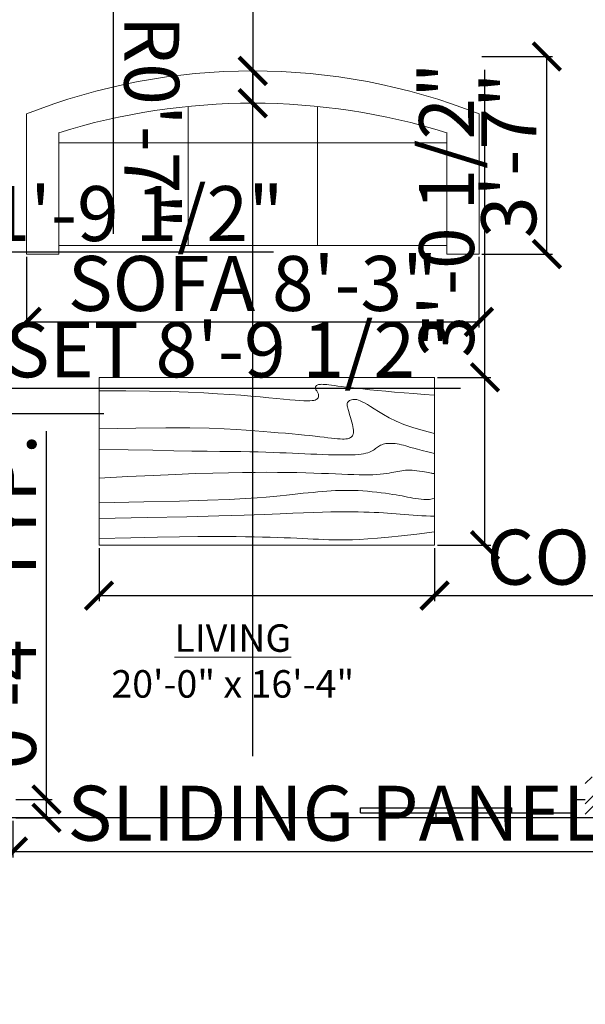
# Model space of a CAD drawing. Units: inches. Extents: x 982 to 1904, y 735 to 1463.
# Tile 5 of 7: x 1566 to 1689, y 945 to 1160. Entities that reach past the tile are written whole.
import ezdxf

# ---------------------------------------------------------------- set-up
doc = ezdxf.new("R2010")
doc.units = ezdxf.units.IN
for name, color, linetype, lineweight in [('A-AREA-IDEN', 7, 'Continuous', 18), ('A-FLOR', 7, 'Continuous', 25), ('Dimensions', 9, 'Continuous', 18), ('Doors', 130, 'Continuous', 25), ('Furniture', 31, 'Continuous', 18), ('Wall Hatch', 23, 'Continuous', 13)]:
    doc.layers.add(name, color=color, linetype=linetype, lineweight=lineweight)
doc.styles.get("Standard").update_dxf_attribs({"font": 'arial.ttf'})
doc.dimstyles.new('ISO-25', dxfattribs={"dimtxt": 12, "dimasz": 6, "dimexe": 1.25, "dimexo": 0.625, "dimtad": 1, "dimlunit": 3, "dimtxsty": 'Standard', "dimblk": 'ARCHTICK', "dimcen": 2.5, "dimadec": 0, "dimazin": 0, "dimtfac": 1, "dimtmove": 0, "dimatfit": 3, "dimfxl": 1, "dimarcsym": 0})

# ---------------------------------------------------------------- blocks, each defined once
blk = doc.blocks.new('Sofa - Roundback 7 ft.')
for p, q in [((-12.00002, -32.4421), (-12.00003, -6.5971)), ((11.99997, -32.4421), (11.99998, -6.5971)), ((-36.000027, -34), (-36.000027, -11.4696)), ((35.99998, -34), (35.99998, -11.4696)), ((-35.999844, -13.3819), (35.9998, -13.3819)), ((-36.000027, -32.4421), (35.99998, -32.4421))]:
    blk.add_line(p, q)
for points in [[(-36.000027, -34), (-42.000027, -34), (-42.000027, -8)], [(41.99998, -8), (41.99998, -34), (35.99998, -34)]]:
    blk.add_lwpolyline(points)
for centre, radius, start, end in [((0, -114.25), 114.25, 68.43141, 111.5686), ((-0.00001, -127.1968), 121.1968, 72.72033, 107.2797)]:
    blk.add_arc(centre, radius, start, end)
blk = doc.blocks.new('Table - Rectangular Woodgrain 60 x 30 in.')
for p, q in [((0, 0), (0, -30)), ((60, 0), (0, 0)), ((60, -30), (60, 0)), ((0, -30), (60, -30))]:
    blk.add_line(p, q)
for points in [[(0, -2.4), (4.8155, -2.418), (9.0302, -2.4688), (12.709, -2.5477), (15.9167, -2.65), (18.7181, -2.7711), (21.1781, -2.9063), (23.3616, -3.0508), (25.3333, -3.2), (27.1477, -3.3495), (28.8172, -3.4958), (30.3437, -3.636), (31.7291, -3.7667), (32.9756, -3.8849), (34.0849, -3.9875), (35.059, -4.0714), (35.9, -4.1334), (36.6114, -4.1711), (37.2041, -4.1854), (37.6906, -4.1779), (38.0833, -4.15), (38.3948, -4.1034), (38.6375, -4.0396), (38.8239, -3.9602), (38.9666, -3.8667), (39.0764, -3.7608), (39.1573, -3.6448), (39.2116, -3.521), (39.2416, -3.3917), (39.2498, -3.2593), (39.2385, -3.1261), (39.21, -2.9944), (39.1666, -2.8667), (39.111, -2.7447), (39.0468, -2.6281), (38.978, -2.5163), (38.9083, -2.4083), (38.8418, -2.3035), (38.7823, -2.201), (38.7337, -2.1001), (38.7, -2), (38.6844, -1.9003), (38.6875, -1.8021), (38.7094, -1.707), (38.75, -1.6167), (38.8094, -1.5326), (38.8875, -1.4563), (38.9844, -1.3893), (39.1, -1.3333), (39.2351, -1.2896), (39.3937, -1.2583), (39.5804, -1.2396), (39.8, -1.2333), (40.057, -1.2396), (40.3562, -1.2583), (40.7023, -1.2896), (41.1, -1.3333), (41.5547, -1.3895), (42.0755, -1.4573), (42.6721, -1.5361), (43.3542, -1.625), (44.1316, -1.7233), (45.014, -1.8302), (46.0114, -1.9449), (47.1333, -2.0667), (48.3862, -2.1947), (49.7625, -2.3281), (51.2513, -2.4663), (52.8416, -2.6083), (54.5226, -2.7535), (56.2833, -2.9011), (58.1127, -3.0501), (60, -3.2)], [(0, -9.2), (6.5759, -9.0858), (11.9385, -9.0365), (16.2527, -9.0418), (19.6833, -9.0917), (22.3952, -9.1759), (24.5531, -9.2844), (26.322, -9.4069), (27.8666, -9.5333), (29.3241, -9.6553), (30.7203, -9.7719), (32.0532, -9.8837), (33.3208, -9.9917), (34.5213, -10.0965), (35.6526, -10.199), (36.7128, -10.2999), (37.7, -10.4), (38.6129, -10.4996), (39.4531, -10.5969), (40.223, -10.6895), (40.925, -10.775), (41.5613, -10.8512), (42.1344, -10.9156), (42.6465, -10.966), (43.1, -11), (43.4976, -11.0158), (43.8437, -11.0136), (44.143, -10.9942), (44.4, -10.9583), (44.6195, -10.9069), (44.8062, -10.8406), (44.9648, -10.7603), (45.1, -10.6667), (45.2155, -10.5598), (45.3114, -10.4365), (45.3871, -10.2929), (45.4416, -10.125), (45.4743, -9.929), (45.4844, -9.7011), (45.4709, -9.4371), (45.4333, -9.1333), (45.3716, -8.7883), (45.2896, -8.4104), (45.1919, -8.0107), (45.0833, -7.6), (44.9685, -7.1893), (44.8521, -6.7896), (44.7388, -6.4117), (44.6333, -6.0667), (44.54, -5.7628), (44.4614, -5.4979), (44.4001, -5.2675), (44.3583, -5.0667), (44.3384, -4.8909), (44.3427, -4.7354), (44.3736, -4.5956), (44.4333, -4.4667), (44.5236, -4.3453), (44.6427, -4.2333), (44.7884, -4.1339), (44.9583, -4.05), (45.1501, -3.9849), (45.3614, -3.9417), (45.59, -3.9234), (45.8333, -3.9333), (46.0915, -3.9749), (46.3734, -4.0531), (46.6906, -4.1736), (47.0542, -4.3417), (47.4756, -4.5629), (47.9661, -4.8427), (48.5372, -5.1866), (49.2, -5.6), (49.9676, -6.0844), (50.8594, -6.625), (51.8965, -7.2031), (53.1, -7.8), (54.491, -8.3969), (56.0906, -8.975), (57.9199, -9.5156), (60, -10)], [(0, -12.8), (5.1847, -12.9322), (9.6213, -13.0323), (13.3963, -13.1059), (16.5958, -13.1583), (19.3063, -13.1952), (21.614, -13.2219), (23.6054, -13.2439), (25.3666, -13.2667), (26.9728, -13.2947), (28.4531, -13.3281), (29.8256, -13.3663), (31.1083, -13.4083), (32.3191, -13.4535), (33.476, -13.501), (34.597, -13.5501), (35.7, -13.6), (36.7984, -13.6497), (37.8875, -13.6979), (38.9578, -13.743), (40, -13.7833), (41.0047, -13.8174), (41.9625, -13.8438), (42.864, -13.8607), (43.7, -13.8667), (44.4631, -13.8604), (45.1552, -13.8417), (45.7801, -13.8104), (46.3416, -13.7667), (46.8439, -13.7104), (47.2906, -13.6417), (47.6858, -13.5604), (48.0333, -13.4667), (48.3375, -13.3608), (48.6042, -13.2448), (48.8396, -13.121), (49.05, -12.9917), (49.2417, -12.8593), (49.4208, -12.7261), (49.5937, -12.5944), (49.7667, -12.4667), (49.9452, -12.3451), (50.1323, -12.2313), (50.3303, -12.1268), (50.5416, -12.0333), (50.7686, -11.9524), (51.0135, -11.8854), (51.2788, -11.8341), (51.5666, -11.8), (51.8785, -11.7843), (52.2116, -11.7865), (52.562, -11.8059), (52.926, -11.8417), (53.2998, -11.8931), (53.6795, -11.9594), (54.0614, -12.0397), (54.4416, -12.1333), (54.8223, -12.2401), (55.2293, -12.3625), (55.6942, -12.5037), (56.2489, -12.6667), (56.9251, -12.8547), (57.7545, -13.0708), (58.7689, -13.3182), (60, -13.6)], [(0, -18), (5.124, -17.7273), (9.6609, -17.5057), (13.6705, -17.3303), (17.2125, -17.1958), (20.3467, -17.0973), (23.1328, -17.0297), (25.6307, -16.9878), (27.9, -16.9667), (29.9928, -16.9617), (31.9302, -16.9703), (33.7254, -16.9907), (35.3917, -17.0208), (36.9423, -17.0588), (38.3906, -17.1026), (39.7499, -17.1503), (41.0333, -17.2), (42.2519, -17.2496), (43.4073, -17.2969), (44.4986, -17.3395), (45.525, -17.375), (46.4858, -17.4012), (47.3802, -17.4156), (48.2074, -17.416), (48.9667, -17.4), (49.6583, -17.3662), (50.2872, -17.3167), (50.8595, -17.2547), (51.3812, -17.1833), (51.8584, -17.1057), (52.2971, -17.025), (52.7034, -16.9443), (53.0833, -16.8667), (53.443, -16.7951), (53.789, -16.7313), (54.128, -16.6768), (54.4666, -16.6334), (54.8115, -16.6024), (55.1693, -16.5854), (55.5465, -16.5841), (55.95, -16.6), (56.3828, -16.6337), (56.8346, -16.6823), (57.2915, -16.7418), (57.7396, -16.8084), (58.165, -16.878), (58.5539, -16.9469), (58.8924, -17.0111), (59.1666, -17.0667), (59.3679, -17.1107), (59.5078, -17.1438), (59.6032, -17.1675), (59.6708, -17.1833), (59.7275, -17.193), (59.7901, -17.1979), (59.8753, -17.1998), (60, -17.2)], [(0, -22.4), (8.0098, -22.2501), (14.4094, -22.1011), (19.4168, -21.9535), (23.25, -21.8083), (26.1269, -21.6663), (28.2656, -21.5281), (29.884, -21.3947), (31.2, -21.2667), (32.3967, -21.1448), (33.5172, -21.0292), (34.5697, -20.9198), (35.5625, -20.8167), (36.5037, -20.7198), (37.4015, -20.6292), (38.2642, -20.5448), (39.1, -20.4667), (39.9164, -20.3951), (40.7187, -20.3313), (41.5117, -20.2768), (42.3, -20.2333), (43.0883, -20.2024), (43.8812, -20.1854), (44.6836, -20.1841), (45.5, -20.2), (46.3328, -20.234), (47.1747, -20.2844), (48.0163, -20.3488), (48.8479, -20.425), (49.66, -20.5106), (50.4429, -20.6031), (51.1872, -20.7004), (51.8833, -20.8), (52.5246, -20.8999), (53.1166, -20.9995), (53.6681, -21.0983), (54.1875, -21.1958), (54.6834, -21.2919), (55.1646, -21.3859), (55.6394, -21.4777), (56.1167, -21.5667), (56.6028, -21.6515), (57.0961, -21.7266), (57.5929, -21.7852), (58.0896, -21.8208), (58.5823, -21.8268), (59.0674, -21.7964), (59.5412, -21.723), (60, -21.6)], [(0, -25.2), (8.6355, -25.0504), (15.7026, -24.9031), (21.4049, -24.7606), (25.9458, -24.625), (29.529, -24.4988), (32.3578, -24.3844), (34.6359, -24.284), (36.5667, -24.2), (38.3213, -24.1341), (39.9417, -24.0854), (41.437, -24.0523), (42.8167, -24.0333), (44.0901, -24.0268), (45.2667, -24.0313), (46.3557, -24.0451), (47.3667, -24.0667), (48.309, -24.0947), (49.1928, -24.1287), (50.0284, -24.168), (50.826, -24.2125), (51.5959, -24.2617), (52.3483, -24.3151), (53.0935, -24.3725), (53.8417, -24.4334), (54.6009, -24.497), (55.3699, -24.561), (56.1454, -24.6226), (56.9239, -24.6792), (57.7021, -24.7279), (58.4764, -24.7662), (59.2435, -24.7911), (60, -24.8)], [(0, -28.8), (5.6867, -28.6681), (10.45, -28.5698), (14.407, -28.5012), (17.675, -28.4584), (20.3711, -28.4374), (22.6125, -28.4344), (24.5164, -28.4455), (26.2, -28.4667), (27.762, -28.4947), (29.2276, -28.5281), (30.6033, -28.5663), (31.8958, -28.6084), (33.1118, -28.6535), (34.2578, -28.7011), (35.3405, -28.7501), (36.3666, -28.8), (37.3443, -28.8497), (38.288, -28.8974), (39.2137, -28.9412), (40.1375, -28.9792), (41.0753, -29.0093), (42.0432, -29.0297), (43.0572, -29.0384), (44.1333, -29.0333), (45.2936, -29.0114), (46.5843, -28.9641), (48.0579, -28.8816), (49.7666, -28.7542), (51.7629, -28.5721), (54.0989, -28.3255), (56.8272, -28.0048), (60, -27.6)]]:
    blk.add_lwpolyline(points)
blk = doc.blocks.new('DOOR-SLIDING-PANEL')
for p, q in [((2, 4), (0, 4)), ((2, 0), (2, 4)), ((49.05, 2.21), (16.06, 2.21)), ((16.06, 1.11), (16.06, 2.21)), ((49.05, 1.11), (49.05, 2.21)), ((49.05, 1.11), (2, 1.11)), ((32.55, 0), (32.55, 1.11))]:
    blk.add_line(p, q)
blk = doc.blocks.new('_ArchTick')
at = {"color": 0, "linetype": 'ByBlock', "const_width": 0.15}
blk.add_lwpolyline([(-0.5, -0.5), (0.5, 0.5)], dxfattribs=at)
blk = doc.blocks.new('*D38')
at = {"layer": 'Defpoints', "color": 0, "transparency": 16777216}
for p in [(1515.5, 985.99), (1564.55, 985.99), (1564.55, 978.63)]:
    blk.add_point(p, dxfattribs=at)
at = {"layer": 'Dimensions', "color": 0, "lineweight": -2, "transparency": 16777216}
for p, q in [((1515.5, 985.37), (1515.5, 977.38)), ((1564.55, 985.37), (1564.55, 977.38)), ((1515.5, 978.63), (1564.55, 978.63)), ((1564.55, 978.63), (1776.25, 978.63))]:
    blk.add_line(p, q, dxfattribs=at)
at = {"layer": 'Dimensions', "color": 0, "lineweight": -2, "transparency": 16777216, "xscale": 6, "yscale": 6, "zscale": 6, "rotation": 180}
blk.add_blockref('_ArchTick', (1515.5, 978.63), dxfattribs=at)
at = {"layer": 'Dimensions', "color": 0, "lineweight": -2, "transparency": 16777216, "xscale": 6, "yscale": 6, "zscale": 6}
blk.add_blockref('_ArchTick', (1564.55, 978.63), dxfattribs=at)
at = {"layer": 'Dimensions', "color": 0, "transparency": 16777216, "insert": (1673.4, 985.46), "char_height": 12, "attachment_point": 5}
blk.add_mtext('SLIDING PANEL 4\'-1" TYP.', dxfattribs=at)
blk = doc.blocks.new('*D39')
at = {"layer": 'Defpoints', "color": 0, "transparency": 16777216}
for p in [(1564.55, 989.99), (1571.9, 989.99), (1564.55, 985.99)]:
    blk.add_point(p, dxfattribs=at)
at = {"layer": 'Dimensions', "color": 0, "lineweight": -2, "transparency": 16777216}
for p, q in [((1571.9, 989.99), (1571.9, 1070.39)), ((1565.17, 989.99), (1573.15, 989.99)), ((1571.9, 985.99), (1571.9, 989.99)), ((1565.17, 985.99), (1573.15, 985.99))]:
    blk.add_line(p, q, dxfattribs=at)
at = {"layer": 'Dimensions', "color": 0, "lineweight": -2, "transparency": 16777216, "xscale": 6, "yscale": 6, "zscale": 6}
for p, rotation in [((1571.9, 989.99), 90), ((1571.9, 985.99), 270)]:
    blk.add_blockref('_ArchTick', p, dxfattribs=dict(at, rotation=rotation))
at = {"layer": 'Dimensions', "color": 0, "transparency": 16777216, "insert": (1565.15, 1033.19), "char_height": 12, "attachment_point": 5, "rotation": 90}
blk.add_mtext('0\'-4" TYP.', dxfattribs=at)
blk = doc.blocks.new('*D40')
at = {"layer": 'Defpoints', "color": 0, "transparency": 16777216}
for p in [(1389.84, 1095.57), (1495.17, 1095.57), (1495.17, 1079.77)]:
    blk.add_point(p, dxfattribs=at)
at = {"layer": 'Dimensions', "color": 0, "lineweight": -2, "transparency": 16777216}
for p, q in [((1389.84, 1094.94), (1389.84, 1078.52)), ((1495.17, 1094.94), (1495.17, 1078.52)), ((1389.84, 1079.77), (1495.17, 1079.77)), ((1495.17, 1079.77), (1662.27, 1079.77))]:
    blk.add_line(p, q, dxfattribs=at)
at = {"layer": 'Dimensions', "color": 0, "lineweight": -2, "transparency": 16777216, "xscale": 6, "yscale": 6, "zscale": 6, "rotation": 180}
blk.add_blockref('_ArchTick', (1389.84, 1079.77), dxfattribs=at)
at = {"layer": 'Dimensions', "color": 0, "lineweight": -2, "transparency": 16777216, "xscale": 6, "yscale": 6, "zscale": 6}
blk.add_blockref('_ArchTick', (1495.17, 1079.77), dxfattribs=at)
at = {"layer": 'Dimensions', "color": 0, "transparency": 16777216, "insert": (1581.72, 1086.6), "char_height": 12, "attachment_point": 5}
blk.add_mtext('DINING SET 8\'-9 1/2"', dxfattribs=at)
blk = doc.blocks.new('*D42')
at = {"layer": 'Defpoints', "color": 0, "transparency": 16777216}
for p in [(1567.53, 1109.05), (1666.29, 1109.05), (1666.29, 1094.24)]:
    blk.add_point(p, dxfattribs=at)
at = {"layer": 'Dimensions', "color": 0, "lineweight": -2, "transparency": 16777216}
for p, q in [((1567.53, 1108.43), (1567.53, 1092.99)), ((1666.29, 1108.43), (1666.29, 1092.99)), ((1567.53, 1094.24), (1666.29, 1094.24))]:
    blk.add_line(p, q, dxfattribs=at)
at = {"layer": 'Dimensions', "color": 0, "lineweight": -2, "transparency": 16777216, "xscale": 6, "yscale": 6, "zscale": 6, "rotation": 180}
blk.add_blockref('_ArchTick', (1567.53, 1094.24), dxfattribs=at)
at = {"layer": 'Dimensions', "color": 0, "lineweight": -2, "transparency": 16777216, "xscale": 6, "yscale": 6, "zscale": 6}
blk.add_blockref('_ArchTick', (1666.29, 1094.24), dxfattribs=at)
at = {"layer": 'Dimensions', "color": 0, "transparency": 16777216, "insert": (1616.91, 1101.08), "char_height": 12, "attachment_point": 5}
blk.add_mtext('SOFA 8\'-3"', dxfattribs=at)
blk = doc.blocks.new('*D43')
at = {"layer": 'Defpoints', "color": 0, "transparency": 16777216}
for p in [(1666.29, 1152.16), (1681.11, 1152.16), (1666.29, 1109.05)]:
    blk.add_point(p, dxfattribs=at)
at = {"layer": 'Dimensions', "color": 0, "lineweight": -2, "transparency": 16777216}
for p, q in [((1666.92, 1152.16), (1682.36, 1152.16)), ((1681.11, 1109.05), (1681.11, 1152.16)), ((1666.92, 1109.05), (1682.36, 1109.05))]:
    blk.add_line(p, q, dxfattribs=at)
at = {"layer": 'Dimensions', "color": 0, "lineweight": -2, "transparency": 16777216, "xscale": 6, "yscale": 6, "zscale": 6}
for p, rotation in [((1681.11, 1152.16), 90), ((1681.11, 1109.05), 270)]:
    blk.add_blockref('_ArchTick', p, dxfattribs=dict(at, rotation=rotation))
at = {"layer": 'Dimensions', "color": 0, "transparency": 16777216, "insert": (1674.35, 1130.61), "char_height": 12, "attachment_point": 5, "rotation": 90}
blk.add_mtext('3\'-7"', dxfattribs=at)
blk = doc.blocks.new('*D46')
at = {"layer": 'Defpoints', "color": 0, "transparency": 16777216}
for p in [(1583.35, 1045.5), (1656.61, 1045.5), (1656.61, 1034.51)]:
    blk.add_point(p, dxfattribs=at)
at = {"layer": 'Dimensions', "color": 0, "lineweight": -2, "transparency": 16777216}
for p, q in [((1583.35, 1044.87), (1583.35, 1033.26)), ((1656.61, 1044.87), (1656.61, 1033.26)), ((1583.35, 1034.51), (1656.61, 1034.51)), ((1656.61, 1034.51), (1854, 1034.51))]:
    blk.add_line(p, q, dxfattribs=at)
at = {"layer": 'Dimensions', "color": 0, "lineweight": -2, "transparency": 16777216, "xscale": 6, "yscale": 6, "zscale": 6, "rotation": 180}
blk.add_blockref('_ArchTick', (1583.35, 1034.51), dxfattribs=at)
at = {"layer": 'Dimensions', "color": 0, "lineweight": -2, "transparency": 16777216, "xscale": 6, "yscale": 6, "zscale": 6}
blk.add_blockref('_ArchTick', (1656.61, 1034.51), dxfattribs=at)
at = {"layer": 'Dimensions', "color": 0, "transparency": 16777216, "insert": (1758.31, 1041.34), "char_height": 12, "attachment_point": 5}
blk.add_mtext('COFFEE TABLE 6\'-1 1/2"', dxfattribs=at)
blk = doc.blocks.new('*D47')
at = {"layer": 'Defpoints', "color": 0, "transparency": 16777216}
for p in [(1656.61, 1082.13), (1667.6, 1082.13), (1656.61, 1045.5)]:
    blk.add_point(p, dxfattribs=at)
at = {"layer": 'Dimensions', "color": 0, "lineweight": -2, "transparency": 16777216}
for p, q in [((1667.6, 1082.13), (1667.6, 1149.23)), ((1657.24, 1082.13), (1668.85, 1082.13)), ((1667.6, 1045.5), (1667.6, 1082.13)), ((1657.24, 1045.5), (1668.85, 1045.5))]:
    blk.add_line(p, q, dxfattribs=at)
at = {"layer": 'Dimensions', "color": 0, "lineweight": -2, "transparency": 16777216, "xscale": 6, "yscale": 6, "zscale": 6}
for p, rotation in [((1667.6, 1082.13), 90), ((1667.6, 1045.5), 270)]:
    blk.add_blockref('_ArchTick', p, dxfattribs=dict(at, rotation=rotation))
at = {"layer": 'Dimensions', "color": 0, "transparency": 16777216, "insert": (1660.77, 1118.68), "char_height": 12, "attachment_point": 5, "rotation": 90}
blk.add_mtext('3\'-0 1/2"', dxfattribs=at)
blk = doc.blocks.new('*D48')
at = {"layer": 'Defpoints', "color": 0, "transparency": 16777216}
for p in [(1555.46, 1134.17), (1558.68, 1134.17), (1555.46, 1112.72)]:
    blk.add_point(p, dxfattribs=at)
at = {"layer": 'Dimensions', "color": 0, "lineweight": -2, "transparency": 16777216}
for p, q in [((1558.68, 1134.17), (1558.68, 1298.47)), ((1556.09, 1134.17), (1559.93, 1134.17)), ((1558.68, 1112.72), (1558.68, 1134.17)), ((1556.09, 1112.72), (1559.93, 1112.72))]:
    blk.add_line(p, q, dxfattribs=at)
at = {"layer": 'Dimensions', "color": 0, "lineweight": -2, "transparency": 16777216, "xscale": 6, "yscale": 6, "zscale": 6}
for p, rotation in [((1558.68, 1134.17), 90), ((1558.68, 1112.72), 270)]:
    blk.add_blockref('_ArchTick', p, dxfattribs=dict(at, rotation=rotation))
at = {"layer": 'Dimensions', "color": 0, "transparency": 16777216, "insert": (1551.85, 1219.32), "char_height": 12, "attachment_point": 5, "rotation": 90}
blk.add_mtext('END TABLE 1\'-9 1/2"', dxfattribs=at)
blk = doc.blocks.new('*D49')
at = {"layer": 'Defpoints', "color": 0, "transparency": 16777216}
for p in [(1534.01, 1112.72), (1555.46, 1112.72), (1555.46, 1109.5)]:
    blk.add_point(p, dxfattribs=at)
at = {"layer": 'Dimensions', "color": 0, "lineweight": -2, "transparency": 16777216}
for p, q in [((1534.01, 1112.09), (1534.01, 1108.25)), ((1555.46, 1112.09), (1555.46, 1108.25)), ((1534.01, 1109.5), (1555.46, 1109.5)), ((1555.46, 1109.5), (1621.44, 1109.5))]:
    blk.add_line(p, q, dxfattribs=at)
at = {"layer": 'Dimensions', "color": 0, "lineweight": -2, "transparency": 16777216, "xscale": 6, "yscale": 6, "zscale": 6, "rotation": 180}
blk.add_blockref('_ArchTick', (1534.01, 1109.5), dxfattribs=at)
at = {"layer": 'Dimensions', "color": 0, "lineweight": -2, "transparency": 16777216, "xscale": 6, "yscale": 6, "zscale": 6}
blk.add_blockref('_ArchTick', (1555.46, 1109.5), dxfattribs=at)
at = {"layer": 'Dimensions', "color": 0, "transparency": 16777216, "insert": (1591.45, 1116.33), "char_height": 12, "attachment_point": 5}
blk.add_mtext('1\'-9 1/2"', dxfattribs=at)
blk = doc.blocks.new('*D73')
at = {"layer": 'Defpoints', "color": 0, "transparency": 16777216}
for p in [(1616.91, 1141.97), (1616.91, 999.48)]:
    blk.add_point(p, dxfattribs=at)
at = {"layer": 'Dimensions', "color": 0, "lineweight": -2, "transparency": 16777216}
for p in [(1616.91, 1273.09), (1616.91, 999.48)]:
    blk.add_line(p, (1616.91, 1141.97), dxfattribs=at)
at = {"layer": 'Dimensions', "color": 0, "lineweight": -2, "transparency": 16777216, "xscale": 6, "yscale": 6, "zscale": 6, "rotation": 269.9998576619989}
blk.add_blockref('_ArchTick', (1616.91, 1141.97), dxfattribs=at)
at = {"layer": 'Dimensions', "color": 0, "transparency": 16777216, "insert": (1610.08, 1227.47), "char_height": 12, "attachment_point": 5, "rotation": 89.9999}
blk.add_mtext('R11\'-10 1/2"', dxfattribs=at)
blk = doc.blocks.new('*D74')
at = {"layer": 'Defpoints', "color": 0, "transparency": 16777216}
for p in [(1616.91, 1149.03), (1616.91, 1014.7)]:
    blk.add_point(p, dxfattribs=at)
at = {"layer": 'Dimensions', "color": 0, "lineweight": -2, "transparency": 16777216}
for p in [(1616.91, 1270.59), (1616.91, 1014.7)]:
    blk.add_line(p, (1616.91, 1149.03), dxfattribs=at)
at = {"layer": 'Dimensions', "color": 0, "lineweight": -2, "transparency": 16777216, "xscale": 6, "yscale": 6, "zscale": 6, "rotation": 269.9998536992126}
blk.add_blockref('_ArchTick', (1616.91, 1149.03), dxfattribs=at)
at = {"layer": 'Dimensions', "color": 0, "transparency": 16777216, "insert": (1610.08, 1229.63), "char_height": 12, "attachment_point": 5, "rotation": 89.9999}
blk.add_mtext('R11\'-2 1/2"', dxfattribs=at)
blk = doc.blocks.new('*D76')
at = {"layer": 'Defpoints', "color": 0, "transparency": 16777216}
for p in [(1519.04, 1074.16), (1583.2, 1074.16)]:
    blk.add_point(p, dxfattribs=at)
at = {"layer": 'Dimensions', "color": 0, "lineweight": -2, "transparency": 16777216}
for p in [(1458.22, 1074.16), (1583.2, 1074.16)]:
    blk.add_line(p, (1519.04, 1074.16), dxfattribs=at)
at = {"layer": 'Dimensions', "color": 0, "lineweight": -2, "transparency": 16777216, "xscale": 6, "yscale": 6, "zscale": 6, "rotation": 359.9995481306522}
blk.add_blockref('_ArchTick', (1519.04, 1074.16), dxfattribs=at)
at = {"layer": 'Dimensions', "color": 0, "transparency": 16777216, "insert": (1480.54, 1080.88), "char_height": 12, "attachment_point": 5, "rotation": 359.9995}
blk.add_mtext('R5\'-4"', dxfattribs=at)
blk = doc.blocks.new('*D77')
at = {"layer": 'Defpoints', "color": 0, "transparency": 16777216}
for p in [(1525.43, 1074.16), (1584.4, 1074.16)]:
    blk.add_point(p, dxfattribs=at)
at = {"layer": 'Dimensions', "color": 0, "lineweight": -2, "transparency": 16777216}
for p in [(1459.47, 1074.16), (1584.4, 1074.16)]:
    blk.add_line(p, (1525.43, 1074.16), dxfattribs=at)
at = {"layer": 'Dimensions', "color": 0, "lineweight": -2, "transparency": 16777216, "xscale": 6, "yscale": 6, "zscale": 6, "rotation": 0.0004799085174027}
blk.add_blockref('_ArchTick', (1525.43, 1074.16), dxfattribs=at)
at = {"layer": 'Dimensions', "color": 0, "transparency": 16777216, "insert": (1486.45, 1080.81), "char_height": 12, "attachment_point": 5, "rotation": 0.0005}
blk.add_mtext('R4\'-11"', dxfattribs=at)
blk = doc.blocks.new('*D79')
at = {"layer": 'Defpoints', "color": 0, "transparency": 16777216}
for p in [(1586.55, 1203.33), (1586.55, 1196.33)]:
    blk.add_point(p, dxfattribs=at)
at = {"layer": 'Dimensions', "color": 0, "lineweight": -2, "transparency": 16777216}
for p in [(1586.55, 1203.33), (1586.55, 1113.43)]:
    blk.add_line(p, (1586.55, 1196.33), dxfattribs=at)
at = {"layer": 'Dimensions', "color": 0, "lineweight": -2, "transparency": 16777216, "xscale": 6, "yscale": 6, "zscale": 6, "rotation": 90.00372422566393}
blk.add_blockref('_ArchTick', (1586.55, 1196.33), dxfattribs=at)
at = {"layer": 'Dimensions', "color": 0, "transparency": 16777216, "insert": (1593.3, 1148.88), "char_height": 12, "attachment_point": 5, "rotation": 270.0037}
blk.add_mtext('4X R0\'-7"', dxfattribs=at)

msp = doc.modelspace()

# ---------------------------------------------------------------- hatches: boundary and pattern name
at = {"layer": 'Wall Hatch'}
h = msp.add_hatch(dxfattribs=at)
h.set_pattern_fill('ANSI32', color=256, scale=0.5)
h.paths.add_polyline_path([(1165.496, 1065.991), (1271.496, 1065.991), (1271.496, 1071.991), (1218.496, 1071.991), (1218.496, 1238.491), (1262.496, 1238.491), (1262.496, 1244.491), (1218.496, 1244.491), (1218.496, 1330.491), (1298.496, 1330.491), (1298.496, 1244.491), (1292.496, 1244.491), (1292.496, 1238.491), (1298.496, 1238.491), (1298.496, 1221.991), (1304.496, 1221.991), (1304.496, 1224.991), (1374.496, 1224.991), (1374.496, 1230.991), (1304.496, 1230.991), (1304.496, 1251.991), (1310.496, 1251.991), (1310.496, 1257.991), (1304.496, 1257.991), (1304.496, 1385.991), (1328.496, 1385.991), (1328.496, 1394.991), (1295.496, 1394.991), (1295.496, 1339.491), (1209.496, 1339.491), (1209.496, 1071.991), (1156.496, 1071.991), (1156.496, 893.991), (1171.496, 893.991), (1171.496, 902.991), (1165.496, 902.991)])
h.paths.add_polyline_path([(1273.996, 877.991), (1267.996, 877.991), (1267.996, 902.991), (1252.996, 902.991), (1252.996, 893.991), (1258.996, 893.991), (1258.996, 868.991), (1273.996, 868.991)])
h.paths.add_polyline_path([(1370.496, 1052.991), (1361.496, 1052.991), (1361.496, 1046.991), (1355.496, 1046.991), (1355.496, 1040.991), (1361.496, 1040.991), (1361.496, 877.991), (1355.496, 877.991), (1355.496, 868.991), (1361.496, 868.991), (1361.496, 832.991), (1376.313, 832.991), (1491.496, 832.991), (1491.496, 985.991), (1515.496, 985.991), (1515.496, 994.991), (1482.496, 994.991), (1482.496, 841.991), (1370.496, 841.991)])
h.paths.add_polyline_path([(1319.496, 1088.991), (1325.496, 1088.991), (1325.496, 1094.991), (1319.496, 1094.991), (1319.496, 1112.491), (1361.496, 1112.491), (1361.496, 1094.991), (1355.496, 1094.991), (1355.496, 1088.991), (1361.496, 1088.991), (1361.496, 1082.991), (1370.496, 1082.991), (1370.496, 1180.991), (1503.496, 1180.991), (1503.496, 1231.991), (1497.496, 1231.991), (1497.496, 1215.991), (1491.496, 1215.991), (1491.496, 1209.991), (1497.496, 1209.991), (1497.496, 1189.991), (1448.496, 1189.991), (1448.496, 1209.991), (1454.496, 1209.991), (1454.496, 1215.991), (1448.496, 1215.991), (1448.496, 1221.991), (1442.496, 1221.991), (1442.496, 1189.991), (1380.496, 1189.991), (1380.496, 1251.991), (1442.496, 1251.991), (1442.496, 1245.991), (1448.496, 1245.991), (1448.496, 1263.991), (1442.496, 1263.991), (1442.496, 1257.991), (1368.496, 1257.991), (1368.496, 1251.991), (1374.496, 1251.991), (1374.496, 1189.991), (1304.496, 1189.991), (1304.496, 1192.991), (1295.496, 1192.991), (1295.496, 1183.991), (1361.496, 1183.991), (1361.496, 1118.491), (1313.496, 1118.491), (1313.496, 1071.991), (1301.496, 1071.991), (1301.496, 1065.991), (1313.496, 1065.991), (1313.496, 1040.991), (1325.496, 1040.991), (1325.496, 1046.991), (1319.496, 1046.991)])
h.paths.add_polyline_path([(1565.496, 1394.991), (1418.496, 1394.991), (1418.496, 1385.991), (1442.496, 1385.991), (1442.496, 1293.991), (1448.496, 1293.991), (1448.496, 1299.991), (1454.496, 1299.991), (1454.496, 1305.991), (1448.496, 1305.991), (1448.496, 1385.991), (1556.496, 1385.991), (1556.496, 1307.991), (1497.496, 1307.991), (1497.496, 1305.991), (1491.496, 1305.991), (1491.496, 1299.991), (1497.496, 1299.991), (1497.496, 1268.991), (1503.496, 1268.991), (1503.496, 1298.991), (1656.496, 1298.991), (1656.496, 1307.991), (1565.496, 1307.991)])
h.paths.add_polyline_path([(1731.496, 1307.991), (1698.496, 1307.991), (1698.496, 1298.991), (1722.496, 1298.991), (1722.496, 1033.991), (1731.496, 1033.991)])
h.paths.add_polyline_path([(1731.496, 997.991), (1722.496, 997.991), (1722.496, 994.991), (1689.496, 994.991), (1689.496, 985.991), (1731.496, 985.991)])

# ---------------------------------------------------------------- linework, layer by layer
at = {"layer": 'A-FLOR'}
msp.add_line((1732.746, 985.991), (1491.496, 985.991), dxfattribs=at)

# ---------------------------------------------------------------- block references
at = {"layer": 'Doors', "extrusion": (0, 0, -1), "zscale": -1}
msp.add_blockref('DOOR-SLIDING-PANEL', (-1689.497, 985.991), dxfattribs=at)
at = {"layer": 'Furniture'}
for name, p, xscale, yscale, zscale in [('Sofa - Roundback 7 ft.', (1616.913, 1149.029), 1.175746996221043, 1.175746996221043, 1.175746996221043), ('Table - Rectangular Woodgrain 60 x 30 in.', (1583.351, 1082.129), 1.221050194161944, 1.221050194161944, 1.221050194161944)]:
    msp.add_blockref(name, p, dxfattribs=dict(at, xscale=xscale, yscale=yscale, zscale=zscale))

# ---------------------------------------------------------------- texts
at = {"layer": 'A-AREA-IDEN', "insert": (1584.404, 1028.239), "char_height": 6, "attachment_point": 1}
msp.add_mtext_dynamic_manual_height_columns('\\pxqc;{\\fTimes New Roman|b0|i0|c0|p18;\\LLIVING\\P\\l20\'-0" x 16\'-4"}', width=56.30854, gutter_width=12.5, heights=[0], dxfattribs=at)

# ---------------------------------------------------------------- dimensions: what is measured, and where the dimension line sits
at = {"layer": 'Dimensions'}
for base, p1, p2, text, picture, middle in [((1558.678, 1134.173), (1555.46, 1112.72), (1555.46, 1134.173), 'END TABLE <>', '*D48', (1551.848, 1219.322)), ((1571.903, 989.991), (1564.546, 985.991), (1564.546, 989.991), '<> TYP.', '*D39', (1565.151, 1033.189))]:
    dim = msp.add_linear_dim(base=base, p1=p1, p2=p2, angle=90, text=text, dimstyle='ISO-25', override={"dimdec": 1, "dimlfac": 1, "dimrnd": 0, "dimzin": 1, "dimdsep": 46, "dimlunit": 4, "dimfrac": 2}, dxfattribs=at)
    dim.commit()
    dim.dimension.update_dxf_attribs({"geometry": picture, "text_midpoint": middle})
for center, mpoint, picture, middle in [((1616.913, 999.478), (1616.913, 1141.974), '*D73', (1616.913, 1227.473)), ((1616.913, 1014.7), (1616.913, 1149.029), '*D74', (1616.913, 1229.626)), ((1583.196, 1074.156), (1519.036, 1074.157), '*D76', (1480.541, 1074.157))]:
    dim = msp.add_radius_dim(center=center, mpoint=mpoint, dimstyle='ISO-25', override={"dimdec": 1, "dimlfac": 1, "dimrnd": 0, "dimzin": 1, "dimdsep": 46, "dimlunit": 4, "dimfrac": 2}, dxfattribs=at)
    dim.commit()
    dim.dimension.update_dxf_attribs({"geometry": picture, "text_midpoint": middle, "dimtype": 164})
dim = msp.add_radius_dim(center=(1586.547, 1203.328), mpoint=(1586.547, 1196.328), text='4X <>', dimstyle='ISO-25', override={"dimdec": 1, "dimlfac": 1, "dimrnd": 0, "dimzin": 1, "dimdsep": 46, "dimlunit": 4, "dimfrac": 2}, dxfattribs=at)
dim.commit()
dim.dimension.update_dxf_attribs({"geometry": '*D79', "text_midpoint": (1593.302, 1148.878)})
for base, p1, p2, picture, middle in [((1681.108, 1152.164), (1666.294, 1109.054), (1666.294, 1152.164), '*D43', (1674.352, 1130.609)), ((1667.604, 1082.129), (1656.614, 1045.497), (1656.614, 1082.129), '*D47', (1660.77, 1118.68))]:
    dim = msp.add_linear_dim(base=base, p1=p1, p2=p2, angle=90, dimstyle='ISO-25', override={"dimdec": 1, "dimlfac": 1, "dimrnd": 0, "dimzin": 1, "dimdsep": 46, "dimlunit": 4, "dimfrac": 2}, dxfattribs=at)
    dim.commit()
    dim.dimension.update_dxf_attribs({"geometry": picture, "text_midpoint": middle})
dim = msp.add_linear_dim(base=(1555.46, 1109.502), p1=(1534.008, 1112.72), p2=(1555.46, 1112.72), dimstyle='ISO-25', override={"dimdec": 1, "dimlfac": 1, "dimrnd": 0, "dimzin": 1, "dimdsep": 46, "dimlunit": 4, "dimfrac": 2}, dxfattribs=at)
dim.commit()
dim.dimension.update_dxf_attribs({"geometry": '*D49', "text_midpoint": (1591.451, 1116.332)})
for base, p1, p2, text, picture, middle in [((1495.169, 1079.77), (1389.84, 1095.569), (1495.169, 1095.569), 'DINING SET <>', '*D40', (1581.722, 1086.6)), ((1666.294, 1094.239), (1567.531, 1109.054), (1666.294, 1109.054), 'SOFA <>', '*D42', (1616.913, 1101.077)), ((1656.614, 1034.508), (1583.351, 1045.497), (1656.614, 1045.497), 'COFFEE TABLE <>', '*D46', (1758.306, 1041.342)), ((1564.5456, 978.6336), (1515.4964, 985.991), (1564.5456, 985.991), 'SLIDING PANEL <> TYP.', '*D38', (1673.3957, 985.4632))]:
    dim = msp.add_linear_dim(base=base, p1=p1, p2=p2, text=text, dimstyle='ISO-25', override={"dimdec": 1, "dimlfac": 1, "dimrnd": 0, "dimzin": 1, "dimdsep": 46, "dimlunit": 4, "dimfrac": 2}, dxfattribs=at)
    dim.commit()
    dim.dimension.update_dxf_attribs({"geometry": picture, "text_midpoint": middle})
dim = msp.add_radius_dim(center=(1584.404, 1074.156), mpoint=(1525.426, 1074.156), dimstyle='ISO-25', override={"dimdec": 1, "dimlfac": 1, "dimrnd": 0, "dimzin": 1, "dimdsep": 46, "dimlunit": 4, "dimfrac": 2}, dxfattribs=at)
dim.commit()
dim.dimension.update_dxf_attribs({"geometry": '*D77', "text_midpoint": (1486.447, 1080.805)})

doc.saveas('drawing.dxf')
